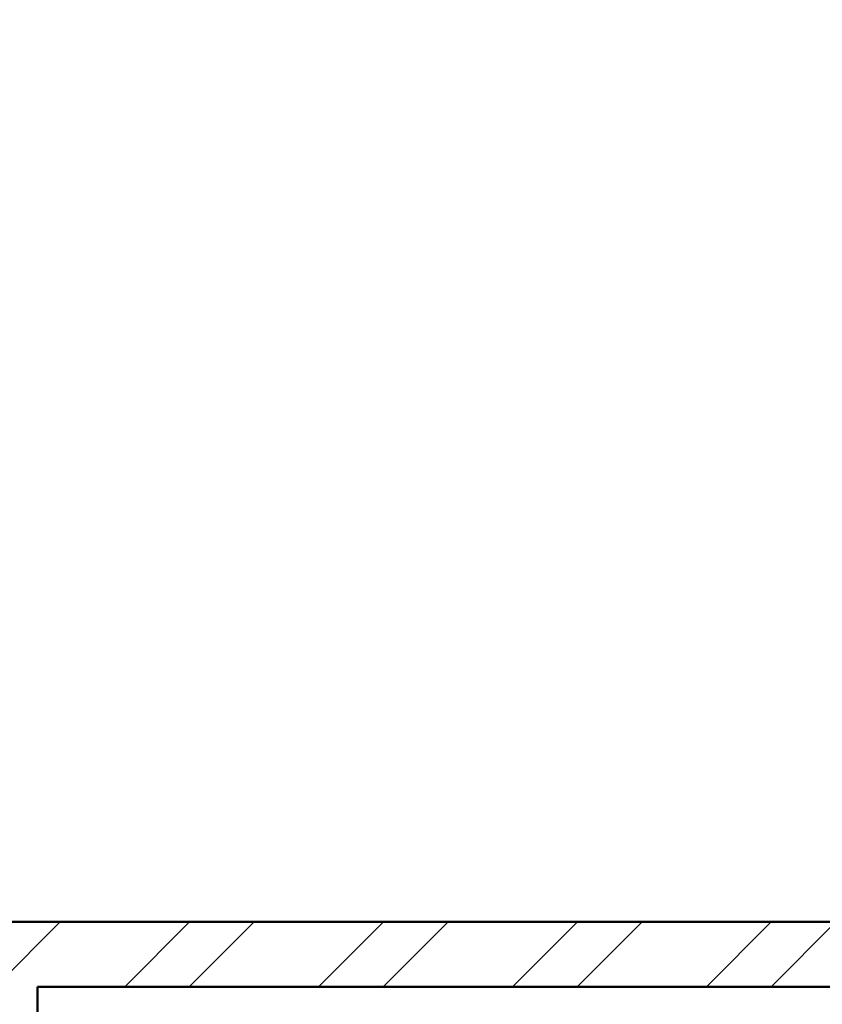
# Model space of a CAD drawing. Units: inches. Extents: x 963 to 2075, y 289 to 2657.
# Tile 69 of 98: x 1399 to 1455, y 2160 to 2228. Entities that reach past the tile are written whole.
import ezdxf

# ---------------------------------------------------------------- set-up
doc = ezdxf.new("R2010")
doc.units = ezdxf.units.IN
doc.layers.add('A-WALL', color=7, linetype='Continuous', lineweight=50)
doc.layers.add('A-WALL-PATT', color=8, linetype='Continuous', lineweight=13)

msp = doc.modelspace()

# ---------------------------------------------------------------- hatches: boundary and pattern name
at = {"layer": 'A-WALL-PATT'}
h = msp.add_hatch(dxfattribs=at)
h.set_pattern_fill('ANSI32', color=256)
h.paths.add_polyline_path([(1473.609, 2163.068), (1473.609, 2165.318), (1376.422, 2165.318), (1376.422, 2227.983), (1371.922, 2227.983), (1371.922, 2214.818), (1368.405, 2214.818), (1368.405, 2210.318), (1371.922, 2210.318), (1371.922, 2160.818), (1395.922, 2160.818), (1395.922, 2090.318), (1217.345, 2090.318), (1217.345, 2085.818), (1395.922, 2085.818), (1458.922, 2085.818), (1458.922, 2108.318), (1454.422, 2108.318), (1454.422, 2090.318), (1400.422, 2090.318), (1400.422, 2160.818), (1473.609, 2160.818)])
h.paths.add_polyline_path([(1649.422, 2210.318), (1653.225, 2210.318), (1653.225, 2214.818), (1649.422, 2214.818), (1649.422, 2227.983), (1644.922, 2227.983), (1644.922, 2165.318), (1550.099, 2165.318), (1550.099, 2160.818), (1620.922, 2160.818), (1620.922, 2112.818), (1555.446, 2112.818), (1555.446, 2108.318), (1584.327, 2108.318), (1584.327, 2084.916), (1588.827, 2084.916), (1588.827, 2108.318), (1625.422, 2108.318), (1667.951, 2108.318), (1667.951, 2022.667), (1588.827, 2022.667), (1588.827, 2047.408), (1584.327, 2047.408), (1584.327, 1996.003), (1588.827, 1996.003), (1588.827, 2018.318), (1667.951, 2018.167), (1667.951, 1928.318), (1625.422, 1928.318), (1625.422, 1923.818), (1672.451, 1923.818), (1672.451, 1928.318), (1672.451, 1946.663), (1785.446, 1946.663), (1785.446, 1951.163), (1743.034, 1951.163), (1743.034, 2017.922), (1841.422, 2017.922), (1841.422, 2014.775), (1845.922, 2014.775), (1845.922, 2017.922), (1905.922, 2017.922), (1905.922, 1987.511), (1910.422, 1987.511), (1910.422, 2022.422), (1910.422, 2068.517), (1905.922, 2068.517), (1905.922, 2022.422), (1845.922, 2022.422), (1845.922, 2025.851), (1843.672, 2025.851), (1841.422, 2025.851), (1841.422, 2022.422), (1743.034, 2022.422), (1743.034, 2084.031), (1768.451, 2084.031), (1785.446, 2084.031), (1785.446, 2088.531), (1672.451, 2088.531), (1672.451, 2112.818), (1667.951, 2112.818), (1625.422, 2112.818), (1625.422, 2160.818), (1649.422, 2160.818)])
h.paths.add_polyline_path([(1672.451, 2084.031), (1738.534, 2084.031), (1738.534, 1951.163), (1672.451, 1951.163)], flags=16)
h.paths.add_polyline_path([(1672.451, 2084.031), (1738.534, 2084.031), (1705.492, 2017.597)], flags=0)
h.paths.add_polyline_path([(1262.766, 2085.818), (1258.266, 2085.818), (1258.266, 2023.278), (1184.422, 2023.278), (1184.422, 2018.778), (1258.266, 2018.778), (1258.266, 1950.818), (1262.766, 1950.818)])
h.paths.add_polyline_path([(1312.266, 2085.818), (1307.766, 2085.818), (1307.766, 1950.818), (1312.266, 1950.818)])
h.paths.add_polyline_path([(1458.922, 1950.818), (1395.922, 1950.818), (1216.568, 1950.818), (1216.568, 1946.318), (1346.422, 1946.318), (1395.922, 1946.318), (1395.922, 1875.818), (1371.922, 1875.818), (1371.922, 1826.318), (1368.931, 1826.318), (1368.931, 1821.818), (1371.922, 1821.818), (1371.922, 1813.622), (1376.422, 1813.622), (1376.422, 1871.318), (1474.504, 1871.318), (1474.504, 1873.568), (1474.504, 1875.818), (1400.422, 1875.818), (1400.422, 1946.318), (1454.422, 1946.318), (1454.422, 1928.318), (1458.922, 1928.318)])
h.paths.add_polyline_path([(1184.422, 2120.778), (1167.922, 2120.778), (1167.922, 2134.812), (1165.672, 2134.812), (1163.422, 2134.812), (1163.422, 2120.778), (1119.922, 2120.778), (1119.922, 2098.095), (1124.422, 2098.095), (1124.422, 2116.278), (1167.922, 2116.278), (1179.922, 2116.278), (1179.922, 2045.916), (1184.422, 2045.916), (1184.422, 2090.318), (1184.422, 2116.278)])
h.paths.add_polyline_path([(1124.422, 2018.778), (1179.922, 2018.778), (1179.922, 2016.294), (1184.422, 2016.294), (1184.422, 2023.278), (1184.422, 2026.588), (1182.172, 2026.588), (1179.922, 2026.588), (1179.922, 2023.278), (1124.422, 2023.278), (1124.422, 2074.095), (1119.922, 2074.095), (1119.922, 2018.778), (1119.922, 1979.633), (1124.422, 1979.633)])
h.paths.add_polyline_path([(1184.422, 1925.778), (1184.422, 1946.318), (1184.422, 1996.073), (1182.172, 1996.073), (1179.922, 1996.073), (1179.922, 1925.778), (1124.422, 1925.778), (1124.422, 1955.633), (1119.922, 1955.502), (1119.922, 1921.278), (1158.922, 1921.278), (1158.922, 1909.983), (1163.422, 1909.983), (1163.422, 1921.278), (1184.422, 1921.278)])
h.paths.add_polyline_path([(1341.449, 1826.318), (1163.422, 1826.318), (1163.422, 1849.983), (1158.922, 1849.983), (1158.922, 1821.818), (1158.922, 1804.033), (1163.422, 1804.033), (1163.422, 1821.818), (1341.449, 1821.818)])
h.paths.add_polyline_path([(1222.981, 1713.818), (1163.422, 1713.818), (1163.422, 1744.033), (1161.172, 1744.033), (1158.922, 1744.033), (1158.922, 1713.818), (1119.922, 1713.818), (1119.922, 1694.65), (1124.422, 1694.65), (1124.422, 1709.318), (1158.922, 1709.318), (1222.981, 1709.318)])
h.paths.add_polyline_path([(1328.422, 1713.818), (1252.042, 1713.818), (1252.042, 1711.568), (1252.042, 1709.318), (1256.422, 1709.318), (1256.422, 1547.318), (1232.937, 1547.318), (1232.937, 1545.068), (1232.937, 1542.818), (1292.422, 1542.818), (1292.422, 1527.634), (1296.922, 1527.634), (1296.922, 1542.818), (1299.464, 1542.818), (1299.464, 1547.318), (1260.922, 1547.318), (1260.922, 1658.318), (1343.661, 1658.318), (1343.661, 1660.568), (1343.661, 1662.818), (1328.422, 1662.818), (1328.422, 1676.589), (1327.402, 1676.589), (1323.922, 1676.589), (1323.922, 1662.818), (1260.922, 1662.818), (1260.922, 1709.318), (1323.922, 1709.318), (1323.922, 1699.851), (1328.422, 1699.851)])
h.paths.add_polyline_path([(1649.422, 1875.818), (1625.422, 1875.818), (1625.422, 1928.318), (1620.922, 1928.318), (1588.827, 1928.318), (1588.827, 1950.59), (1584.327, 1950.59), (1584.327, 1928.318), (1555.446, 1928.318), (1555.446, 1923.818), (1620.922, 1923.818), (1620.922, 1875.818), (1548.952, 1875.818), (1548.952, 1873.568), (1548.952, 1871.318), (1644.922, 1871.318), (1644.922, 1813.622), (1649.422, 1813.622), (1649.422, 1821.818), (1652.045, 1821.818), (1652.045, 1824.068), (1652.045, 1826.318), (1649.422, 1826.318)])
h.paths.add_polyline_path([(1512.922, 1871.318), (1516.476, 1871.318), (1516.476, 1875.818), (1512.922, 1875.818), (1512.922, 1923.818), (1512.922, 1928.318), (1512.922, 1930.827), (1508.422, 1930.827), (1508.422, 1875.818), (1504.411, 1875.818), (1504.411, 1871.318), (1508.422, 1871.318), (1508.422, 1713.818), (1376.422, 1713.818), (1376.422, 1743.325), (1371.922, 1743.325), (1371.922, 1709.318), (1371.922, 1706.01), (1376.422, 1706.01), (1376.422, 1709.318), (1508.422, 1709.318), (1508.422, 1547.318), (1501.871, 1547.318), (1501.871, 1542.818), (1508.422, 1542.818), (1508.422, 1482.818), (1508.422, 1436.318), (1512.922, 1436.318), (1512.922, 1542.818), (1519.318, 1542.818), (1519.318, 1545.068), (1519.318, 1547.318), (1512.922, 1547.318), (1512.922, 1709.318), (1644.922, 1709.318), (1644.922, 1707.548), (1649.422, 1707.548), (1649.422, 1709.318), (1649.422, 1743.325), (1644.922, 1743.325), (1644.922, 1713.818), (1512.922, 1713.818)])
h.paths.add_polyline_path([(1129.884, 1545.068), (1129.884, 1547.318), (1124.422, 1547.318), (1095.922, 1547.318), (1095.922, 1614.818), (1124.422, 1614.818), (1124.422, 1619.318), (1095.922, 1619.318), (1091.422, 1619.318), (1091.422, 1542.818), (1095.922, 1542.818), (1119.922, 1542.818), (1129.884, 1542.818)])
h.paths.add_polyline_path([(1208.422, 1542.818), (1211.74, 1542.818), (1211.74, 1547.318), (1198.851, 1547.318), (1198.851, 1542.818), (1203.922, 1542.818), (1203.922, 1478.318), (1208.422, 1478.318), (1296.922, 1478.318), (1296.922, 1503.634), (1292.422, 1503.634), (1292.422, 1482.818), (1208.422, 1482.818)])
h.paths.add_polyline_path([(1430.422, 1542.818), (1435.699, 1542.818), (1435.699, 1545.068), (1435.699, 1547.318), (1422.658, 1547.318), (1422.658, 1545.068), (1422.658, 1542.818), (1425.922, 1542.818), (1425.922, 1482.857), (1341.922, 1482.857), (1341.922, 1502.732), (1337.422, 1502.732), (1337.422, 1478.357), (1425.922, 1478.357), (1425.922, 1440.818), (1425.922, 1436.318), (1430.422, 1436.318)])
h.paths.add_polyline_path([(1698.482, 2004.259), (1727.695, 2004.259), (1727.695, 2022.916), (1698.482, 2022.916)], flags=8)

# ---------------------------------------------------------------- linework, layer by layer
at = {"layer": 'A-WALL'}
for p, q in [((1376.422, 2165.318), (1475.023, 2165.318)), ((1400.422, 2160.818), (1400.422, 2090.318)), ((1400.422, 2160.818), (1473.609, 2160.818))]:
    msp.add_line(p, q, dxfattribs=at)

doc.saveas('drawing.dxf')
